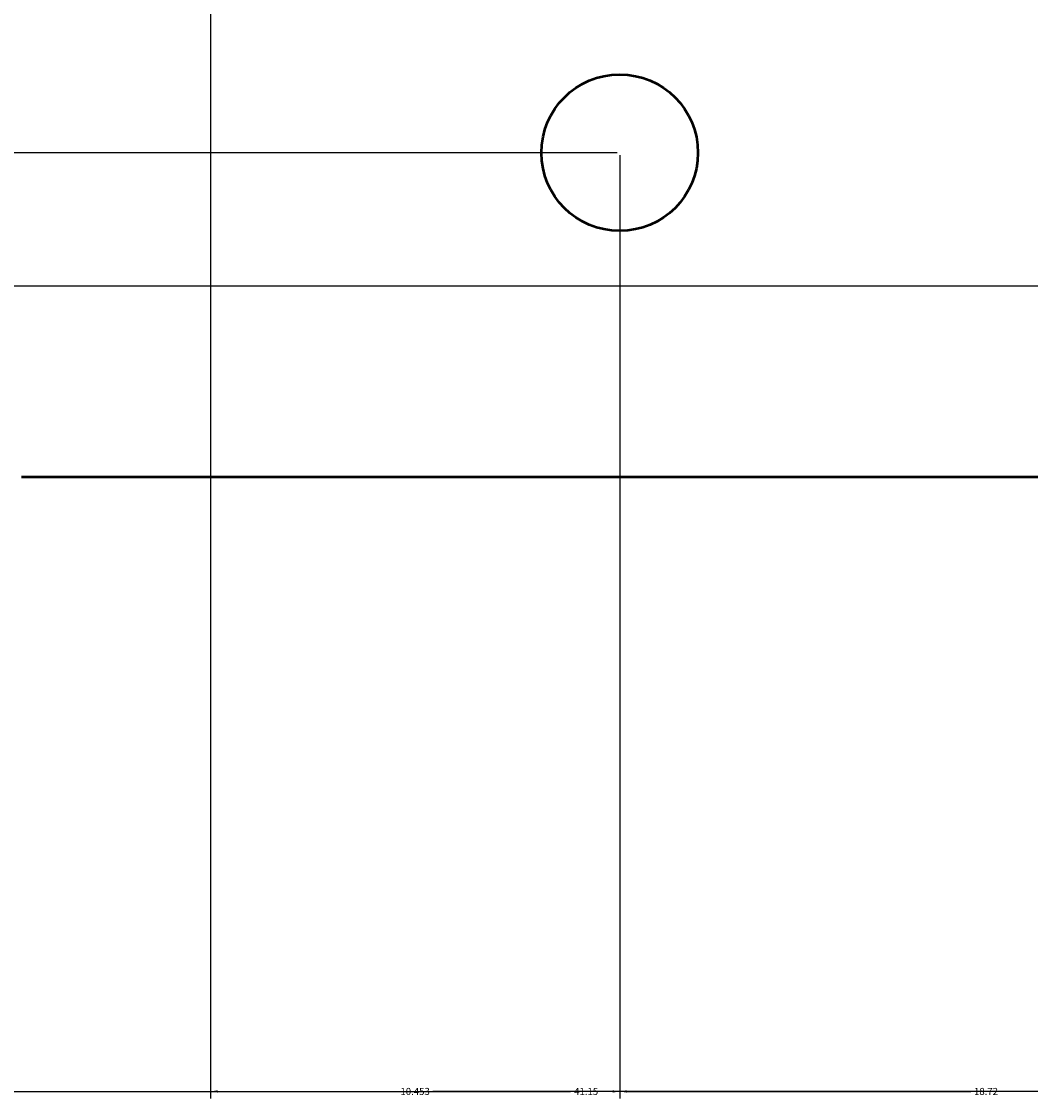
# Model space of a CAD drawing. Units: inches. Extents: x -14 to 108, y -9 to 83.
# Tile 2 of 13: x 12 to 38, y -9 to 19. Entities that reach past the tile are written whole.
import ezdxf

# ---------------------------------------------------------------- set-up
doc = ezdxf.new("R2010")
doc.units = ezdxf.units.IN
doc.header["$MEASUREMENT"] = 0
doc.layers.add('M-DIMS', color=2, linetype='Continuous', lineweight=18)
doc.layers.add('M-OUTL', color=7, linetype='Continuous', lineweight=50)
doc.styles.get("Standard").update_dxf_attribs({"font": 'arial.ttf'})
doc.dimstyles.get("Standard").update_dxf_attribs({"dimtxt": 0.18, "dimasz": 0.18, "dimexe": 0.18, "dimexo": 0.0625, "dimgap": 0.09, "dimtad": 0, "dimtih": 1, "dimtoh": 1, "dimzin": 0, "dimdsep": 46, "dimtxsty": 'Standard', "dimcen": 0.09, "dimadec": 0, "dimazin": 0, "dimtfac": 1, "dimtofl": 0, "dimtmove": 0, "dimatfit": 3, "dimfxl": 1, "dimtolj": 1, "dimtzin": 0, "dimarcsym": 0})

# ---------------------------------------------------------------- blocks, each defined once
blk = doc.blocks.new('HOLE-D4')
blk.add_circle((2, 2), 2)
blk = doc.blocks.new('*D7')
at = {"layer": 'Defpoints', "color": 0, "transparency": 16777216}
for p in [(47.098, 37.119), (5.951, 18.227), (47.098, -8.596)]:
    blk.add_point(p, dxfattribs=at)
at = {"layer": 'M-DIMS', "color": 0, "lineweight": -2, "transparency": 16777216}
for p, q in [((47.098, 37.057), (47.098, -8.776)), ((5.951, 18.165), (5.951, -8.776)), ((6.131, -8.596), (26.126, -8.596)), ((46.918, -8.596), (26.922, -8.596))]:
    blk.add_line(p, q, dxfattribs=at)
at = {"layer": 'M-DIMS', "color": 0, "transparency": 16777216}
for points in [[(6.131, -8.566), (6.131, -8.626), (5.951, -8.596)], [(46.918, -8.566), (46.918, -8.626), (47.098, -8.596)]]:
    blk.add_solid(points, dxfattribs=at)
at = {"layer": 'M-DIMS', "color": 0, "transparency": 16777216, "insert": (26.524, -8.596), "char_height": 0.18, "attachment_point": 5}
blk.add_mtext('\\A1;41.15', dxfattribs=at)
blk = doc.blocks.new('*D16')
at = {"layer": 'Defpoints', "color": 0, "transparency": 16777216}
for p in [(16.928, 37.119), (27.381, 15.402), (27.381, -8.596)]:
    blk.add_point(p, dxfattribs=at)
at = {"layer": 'M-DIMS', "color": 0, "lineweight": -2, "transparency": 16777216}
for p, q in [((16.928, 37.057), (16.928, -8.776)), ((27.381, 15.34), (27.381, -8.776)), ((17.108, -8.596), (21.699, -8.596)), ((27.201, -8.596), (22.61, -8.596))]:
    blk.add_line(p, q, dxfattribs=at)
at = {"layer": 'M-DIMS', "color": 0, "transparency": 16777216}
for points in [[(17.108, -8.566), (17.108, -8.626), (16.928, -8.596)], [(27.201, -8.566), (27.201, -8.626), (27.381, -8.596)]]:
    blk.add_solid(points, dxfattribs=at)
at = {"layer": 'M-DIMS', "color": 0, "transparency": 16777216, "insert": (22.154, -8.596), "char_height": 0.18, "attachment_point": 5}
blk.add_mtext('\\A1;10.453', dxfattribs=at)
blk = doc.blocks.new('*D17')
at = {"layer": 'Defpoints', "color": 0, "transparency": 16777216}
for p in [(27.381, 15.402), (46.1, 11.987), (46.1, -8.596)]:
    blk.add_point(p, dxfattribs=at)
at = {"layer": 'M-DIMS', "color": 0, "lineweight": -2, "transparency": 16777216}
for p, q in [((27.381, 15.34), (27.381, -8.776)), ((46.1, 11.925), (46.1, -8.776)), ((27.561, -8.596), (36.356, -8.596)), ((45.92, -8.596), (37.125, -8.596))]:
    blk.add_line(p, q, dxfattribs=at)
at = {"layer": 'M-DIMS', "color": 0, "transparency": 16777216}
for points in [[(27.561, -8.566), (27.561, -8.626), (27.381, -8.596)], [(45.92, -8.566), (45.92, -8.626), (46.1, -8.596)]]:
    blk.add_solid(points, dxfattribs=at)
at = {"layer": 'M-DIMS', "color": 0, "transparency": 16777216, "insert": (36.741, -8.596), "char_height": 0.18, "attachment_point": 5}
blk.add_mtext('\\A1;18.72', dxfattribs=at)
blk = doc.blocks.new('*D19')
at = {"layer": 'Defpoints', "color": 0, "transparency": 16777216}
for p in [(-13.617, 37.119), (16.928, 37.119), (27.381, 15.402)]:
    blk.add_point(p, dxfattribs=at)
at = {"layer": 'M-DIMS', "color": 0, "lineweight": -2, "transparency": 16777216}
for p, q in [((16.865, 37.119), (-13.797, 37.119)), ((-13.617, 36.939), (-13.617, 26.441)), ((-13.617, 15.582), (-13.617, 26.08)), ((27.318, 15.402), (-13.797, 15.402))]:
    blk.add_line(p, q, dxfattribs=at)
at = {"layer": 'M-DIMS', "color": 0, "transparency": 16777216}
for points in [[(-13.647, 36.939), (-13.587, 36.939), (-13.617, 37.119)], [(-13.647, 15.582), (-13.587, 15.582), (-13.617, 15.402)]]:
    blk.add_solid(points, dxfattribs=at)
at = {"layer": 'M-DIMS', "color": 0, "transparency": 16777216, "insert": (-13.617, 26.261), "char_height": 0.18, "attachment_point": 5}
blk.add_mtext('\\A1;21.717', dxfattribs=at)
blk = doc.blocks.new('*D20')
at = {"layer": 'Defpoints', "color": 0, "transparency": 16777216}
for p in [(-13.617, 15.402), (27.381, 15.402), (46.1, 11.987)]:
    blk.add_point(p, dxfattribs=at)
at = {"layer": 'M-DIMS', "color": 0, "lineweight": -2, "transparency": 16777216}
for p, q in [((27.318, 15.402), (-13.797, 15.402)), ((-13.617, 15.222), (-13.617, 13.877)), ((-13.617, 12.167), (-13.617, 13.513)), ((46.038, 11.987), (-13.797, 11.987))]:
    blk.add_line(p, q, dxfattribs=at)
at = {"layer": 'M-DIMS', "color": 0, "transparency": 16777216}
for points in [[(-13.647, 15.222), (-13.587, 15.222), (-13.617, 15.402)], [(-13.647, 12.167), (-13.587, 12.167), (-13.617, 11.987)]]:
    blk.add_solid(points, dxfattribs=at)
at = {"layer": 'M-DIMS', "color": 0, "transparency": 16777216, "insert": (-13.617, 13.695), "char_height": 0.18, "attachment_point": 5}
blk.add_mtext('\\A1;3.415', dxfattribs=at)

msp = doc.modelspace()

# ---------------------------------------------------------------- linework, layer by layer
at = {"layer": 'M-OUTL'}
msp.add_lwpolyline([(12.0979, 7.1193), (82.0979, 7.1193)], dxfattribs=at)

# ---------------------------------------------------------------- block references
msp.add_blockref('HOLE-D4', (25.381, 13.4019), dxfattribs=at)

# ---------------------------------------------------------------- dimensions: what is measured, and where the dimension line sits
at = {"layer": 'M-DIMS'}
for base, p1, p2, picture, middle in [((-13.6171, 37.1193), (27.3809, 15.4023), (16.9278, 37.1193), '*D19', (-13.6171, 26.2608)), ((-13.6171, 15.4023), (46.1003, 11.987), (27.3809, 15.4023), '*D20', (-13.6171, 13.6947))]:
    dim = msp.add_linear_dim(base=base, p1=p1, p2=p2, angle=90, dimstyle='Standard', override={"dimdec": 3, "dimlfac": 1, "dimrnd": 0, "dimzin": 0, "dimdsep": 46, "dimlunit": 2}, dxfattribs=at)
    dim.commit()
    dim.dimension.update_dxf_attribs({"geometry": picture, "text_midpoint": middle})
for base, p1, p2, override, picture, middle in [((47.0979, -8.5957), (5.9508, 18.2274), (47.0979, 37.1193), {"dimdec": 2, "dimlfac": 1, "dimrnd": 0, "dimzin": 0, "dimdsep": 46, "dimlunit": 2}, '*D7', (26.5244, -8.5957)), ((27.3809, -8.5957), (16.9278, 37.1193), (27.3809, 15.4023), {"dimdec": 3, "dimlfac": 1, "dimrnd": 0, "dimzin": 0, "dimdsep": 46, "dimlunit": 2}, '*D16', (22.1543, -8.5957)), ((46.1003, -8.5957), (27.3809, 15.4023), (46.1003, 11.987), {"dimdec": 2, "dimlfac": 1, "dimrnd": 0, "dimzin": 0, "dimdsep": 46, "dimlunit": 2}, '*D17', (36.7406, -8.5957))]:
    dim = msp.add_linear_dim(base=base, p1=p1, p2=p2, dimstyle='Standard', override=override, dxfattribs=at)
    dim.commit()
    dim.dimension.update_dxf_attribs({"geometry": picture, "text_midpoint": middle})

doc.saveas('drawing.dxf')
